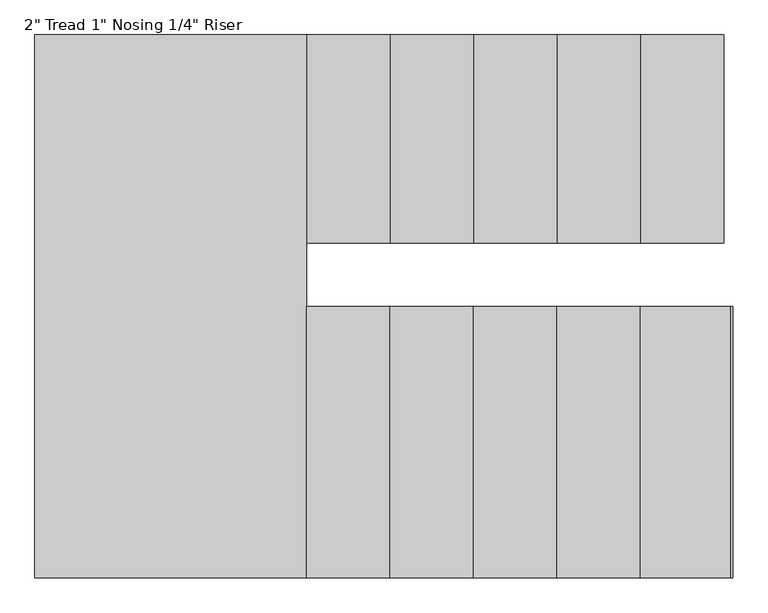
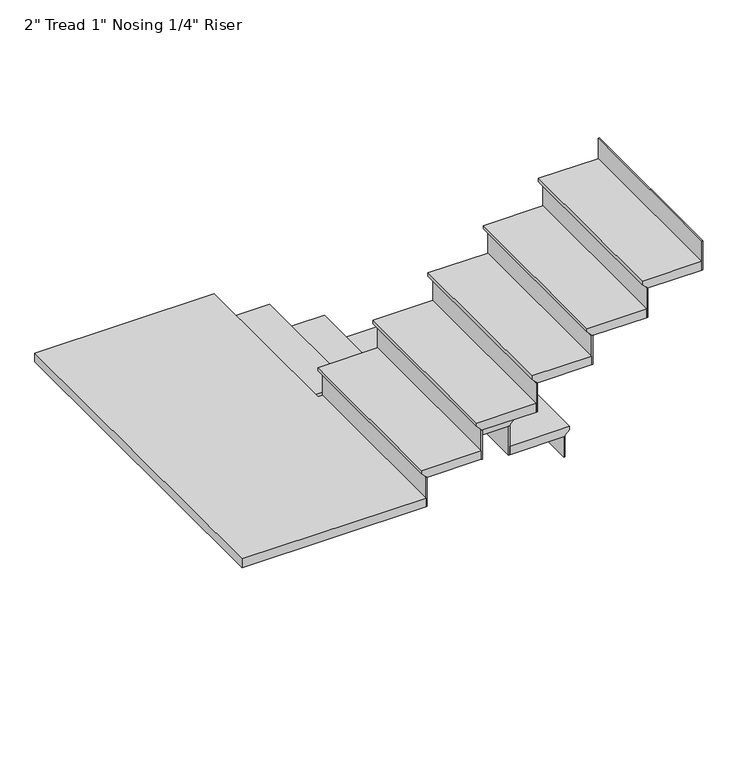
"""IFC4 building model written with IfcOpenShell, lengths in millimetres: stair flight geometry."""

from ifc_helpers import new_model, si_unit, origin, place, context, project, spatial, faceted_brep, source, transform, mapped, element, save


def stair_flight_99d63151(model_context):
    return source(origin(), model_context, "Body", "Brep", [
        faceted_brep([(-3084.0415084, -317.1427733, 9751.4833333), (-3084.0415084, -317.1427733, 9770.5333333), (-3084.0415084, -1076.6758739, 9770.5333333), (-3084.0415084, -1076.6758739, 9751.4833333), (-3109.4415084, -317.1427733, 9726.0833333), (-3109.4415084, -1076.6758739, 9726.0833333), (-3414.2415084, -317.1427733, 9770.5333333), (-3414.2415084, -1076.6758739, 9770.5333333), (-3109.4415084, -1076.6758739, 9719.7333333), (-3414.2415084, -1076.6758739, 9719.7333333), (-3414.2415084, -317.1427733, 9719.7333333), (-3109.4415084, -317.1427733, 9719.7333333)], [[[0, 1, 2, 3]], [[4, 0, 3, 5]], [[2, 1, 6, 7]], [[8, 9, 10, 11]], [[2, 7, 9, 8, 5, 3]], [[8, 11, 4, 5]], [[6, 1, 0, 4, 11, 10]], [[7, 6, 10, 9]]]),
        faceted_brep([(-3109.4415084, -317.1427733, 9719.7333333), (-3109.4415084, -317.1427733, 9601.2), (-3115.7915084, -317.1427733, 9601.2), (-3115.7915084, -317.1427733, 9719.7333333), (-3109.4415084, -1076.6758739, 9719.7333333), (-3115.7915084, -1076.6758739, 9719.7333333), (-3115.7915084, -1076.6758739, 9601.2), (-3109.4415084, -1076.6758739, 9601.2)], [[[0, 1, 2, 3]], [[4, 5, 6, 7]], [[1, 0, 4, 7]], [[2, 1, 7, 6]], [[3, 2, 6, 5]], [[0, 3, 5, 4]]]),
        faceted_brep([(-3414.2415084, -317.1427733, 9889.0666667), (-3414.2415084, -317.1427733, 9719.7333333), (-3420.5915084, -317.1427733, 9719.7333333), (-3420.5915084, -317.1427733, 9889.0666667), (-3414.2415084, -1076.6758739, 9889.0666667), (-3420.5915084, -1076.6758739, 9889.0666667), (-3420.5915084, -1076.6758739, 9719.7333333), (-3414.2415084, -1076.6758739, 9719.7333333)], [[[0, 1, 2, 3]], [[4, 5, 6, 7]], [[1, 0, 4, 7]], [[2, 1, 7, 6]], [[3, 2, 6, 5]], [[0, 3, 5, 4]]]),
        faceted_brep([(-3388.8415084, -1076.6758739, 9939.8666667), (-3388.8415084, -317.1427733, 9939.8666667), (-3719.0415084, -317.1427733, 9939.8666667), (-3719.0415084, -1076.6758739, 9939.8666667), (-3414.2415084, -1076.6758739, 9889.0666667), (-3719.0415084, -1076.6758739, 9889.0666667), (-3719.0415084, -317.1427733, 9889.0666667), (-3414.2415084, -317.1427733, 9889.0666667), (-3414.2415084, -1076.6758739, 9895.4166667), (-3388.8415084, -1076.6758739, 9920.8166667), (-3414.2415084, -317.1427733, 9895.4166667), (-3388.8415084, -317.1427733, 9920.8166667)], [[[0, 1, 2, 3]], [[4, 5, 6, 7]], [[0, 3, 5, 4, 8, 9]], [[4, 7, 10, 8]], [[2, 1, 11, 10, 7, 6]], [[3, 2, 6, 5]], [[11, 1, 0, 9]], [[10, 11, 9, 8]]]),
        faceted_brep([(-3719.0415084, -317.1427733, 10058.4), (-3719.0415084, -317.1427733, 9889.0666667), (-3725.3915084, -317.1427733, 9889.0666667), (-3725.3915084, -317.1427733, 10058.4), (-3719.0415084, -1076.6758739, 10058.4), (-3725.3915084, -1076.6758739, 10058.4), (-3725.3915084, -1076.6758739, 9889.0666667), (-3719.0415084, -1076.6758739, 9889.0666667)], [[[0, 1, 2, 3]], [[4, 5, 6, 7]], [[1, 0, 4, 7]], [[2, 1, 7, 6]], [[3, 2, 6, 5]], [[0, 3, 5, 4]]]),
        faceted_brep([(-3693.6415084, -1076.6758739, 10109.2), (-3693.6415084, -317.1427733, 10109.2), (-4023.8415084, -317.1427733, 10109.2), (-4023.8415084, -1076.6758739, 10109.2), (-3719.0415084, -1076.6758739, 10058.4), (-4023.8415084, -1076.6758739, 10058.4), (-4023.8415084, -317.1427733, 10058.4), (-3719.0415084, -317.1427733, 10058.4), (-3719.0415084, -1076.6758739, 10064.75), (-3693.6415084, -1076.6758739, 10090.15), (-3719.0415084, -317.1427733, 10064.75), (-3693.6415084, -317.1427733, 10090.15)], [[[0, 1, 2, 3]], [[4, 5, 6, 7]], [[0, 3, 5, 4, 8, 9]], [[4, 7, 10, 8]], [[2, 1, 11, 10, 7, 6]], [[3, 2, 6, 5]], [[11, 1, 0, 9]], [[10, 11, 9, 8]]]),
        faceted_brep([(-4023.8415084, -317.1427733, 10227.7333333), (-4023.8415084, -317.1427733, 10058.4), (-4030.1915084, -317.1427733, 10058.4), (-4030.1915084, -317.1427733, 10227.7333333), (-4023.8415084, -1076.6758739, 10227.7333333), (-4030.1915084, -1076.6758739, 10227.7333333), (-4030.1915084, -1076.6758739, 10058.4), (-4023.8415084, -1076.6758739, 10058.4)], [[[0, 1, 2, 3]], [[4, 5, 6, 7]], [[1, 0, 4, 7]], [[2, 1, 7, 6]], [[3, 2, 6, 5]], [[0, 3, 5, 4]]]),
        faceted_brep([(-3998.4415084, -1076.6758739, 10278.5333333), (-3998.4415084, -317.1427733, 10278.5333333), (-4328.6415084, -317.1427733, 10278.5333333), (-4328.6415084, -1076.6758739, 10278.5333333), (-4023.8415084, -1076.6758739, 10227.7333333), (-4328.6415084, -1076.6758739, 10227.7333333), (-4328.6415084, -317.1427733, 10227.7333333), (-4023.8415084, -317.1427733, 10227.7333333), (-4023.8415084, -1076.6758739, 10234.0833333), (-3998.4415084, -1076.6758739, 10259.4833333), (-4023.8415084, -317.1427733, 10234.0833333), (-3998.4415084, -317.1427733, 10259.4833333)], [[[0, 1, 2, 3]], [[4, 5, 6, 7]], [[0, 3, 5, 4, 8, 9]], [[4, 7, 10, 8]], [[2, 1, 11, 10, 7, 6]], [[3, 2, 6, 5]], [[11, 1, 0, 9]], [[10, 11, 9, 8]]]),
        faceted_brep([(-4328.6415084, -317.1427733, 10397.0666667), (-4328.6415084, -317.1427733, 10227.7333333), (-4334.9915084, -317.1427733, 10227.7333333), (-4334.9915084, -317.1427733, 10397.0666667), (-4328.6415084, -1076.6758739, 10397.0666667), (-4334.9915084, -1076.6758739, 10397.0666667), (-4334.9915084, -1076.6758739, 10227.7333333), (-4328.6415084, -1076.6758739, 10227.7333333)], [[[0, 1, 2, 3]], [[4, 5, 6, 7]], [[1, 0, 4, 7]], [[2, 1, 7, 6]], [[3, 2, 6, 5]], [[0, 3, 5, 4]]]),
        faceted_brep([(-4303.2415084, -1076.6758739, 10447.8666667), (-4303.2415084, -317.1427733, 10447.8666667), (-4633.4415084, -317.1427733, 10447.8666667), (-4633.4415084, -1076.6758739, 10447.8666667), (-4328.6415084, -1076.6758739, 10397.0666667), (-4633.4415084, -1076.6758739, 10397.0666667), (-4633.4415084, -317.1427733, 10397.0666667), (-4328.6415084, -317.1427733, 10397.0666667), (-4328.6415084, -1076.6758739, 10403.4166667), (-4303.2415084, -1076.6758739, 10428.8166667), (-4328.6415084, -317.1427733, 10403.4166667), (-4303.2415084, -317.1427733, 10428.8166667)], [[[0, 1, 2, 3]], [[4, 5, 6, 7]], [[0, 3, 5, 4, 8, 9]], [[4, 7, 10, 8]], [[2, 1, 11, 10, 7, 6]], [[3, 2, 6, 5]], [[11, 1, 0, 9]], [[10, 11, 9, 8]]]),
        faceted_brep([(-4633.4415084, -317.1427733, 10566.4), (-4633.4415084, -317.1427733, 10397.0666667), (-4639.7915084, -317.1427733, 10397.0666667), (-4639.7915084, -317.1427733, 10566.4), (-4633.4415084, -1076.6758739, 10566.4), (-4639.7915084, -1076.6758739, 10566.4), (-4639.7915084, -1076.6758739, 10397.0666667), (-4633.4415084, -1076.6758739, 10397.0666667)], [[[0, 1, 2, 3]], [[4, 5, 6, 7]], [[1, 0, 4, 7]], [[2, 1, 7, 6]], [[3, 2, 6, 5]], [[0, 3, 5, 4]]]),
        faceted_brep([(-4582.6415084, -1307.7427733, 10617.2), (-4608.0415084, -1307.7427733, 10617.2), (-4608.0415084, -317.1427733, 10617.2), (-5598.6415084, -317.1427733, 10617.2), (-5598.6415084, -2298.3427733, 10617.2), (-4582.6415084, -2298.3427733, 10617.2), (-4608.0415084, -1307.7427733, 10566.4), (-4582.6415084, -1307.7427733, 10566.4), (-4582.6415084, -2298.3427733, 10566.4), (-5598.6415084, -2298.3427733, 10566.4), (-5598.6415084, -317.1427733, 10566.4), (-4633.4415084, -317.1427733, 10566.4), (-4633.4415084, -1076.6758739, 10566.4), (-4608.0415084, -1076.6758739, 10566.4), (-4608.0415084, -1076.6758739, 10598.15), (-4608.0415084, -317.1427733, 10598.15), (-4633.4415084, -1076.6758739, 10572.75), (-4633.4415084, -317.1427733, 10572.75)], [[[0, 1, 2, 3, 4, 5]], [[6, 7, 8, 9, 10, 11, 12, 13]], [[1, 0, 7, 6]], [[2, 1, 6, 13, 14, 15]], [[13, 12, 16, 14]], [[12, 11, 17, 16]], [[3, 2, 15, 17, 11, 10]], [[4, 3, 10, 9]], [[5, 4, 9, 8]], [[0, 5, 8, 7]], [[17, 15, 14, 16]]]),
        faceted_brep([(-4582.6415084, -2298.3427733, 10735.7333333), (-4582.6415084, -2298.3427733, 10566.4), (-4576.2915084, -2298.3427733, 10566.4), (-4576.2915084, -2298.3427733, 10735.7333333), (-4582.6415084, -1307.7427733, 10735.7333333), (-4576.2915084, -1307.7427733, 10735.7333333), (-4576.2915084, -1307.7427733, 10566.4), (-4582.6415084, -1307.7427733, 10566.4)], [[[0, 1, 2, 3]], [[4, 5, 6, 7]], [[1, 0, 4, 7]], [[2, 1, 7, 6]], [[3, 2, 6, 5]], [[0, 3, 5, 4]]]),
        faceted_brep([(-4608.0415084, -1307.7427733, 10786.5333333), (-4608.0415084, -2298.3427733, 10786.5333333), (-4277.8415084, -2298.3427733, 10786.5333333), (-4277.8415084, -1307.7427733, 10786.5333333), (-4582.6415084, -1307.7427733, 10735.7333333), (-4277.8415084, -1307.7427733, 10735.7333333), (-4277.8415084, -2298.3427733, 10735.7333333), (-4582.6415084, -2298.3427733, 10735.7333333), (-4582.6415084, -1307.7427733, 10742.0833333), (-4608.0415084, -1307.7427733, 10767.4833333), (-4582.6415084, -2298.3427733, 10742.0833333), (-4608.0415084, -2298.3427733, 10767.4833333)], [[[0, 1, 2, 3]], [[4, 5, 6, 7]], [[0, 3, 5, 4, 8, 9]], [[4, 7, 10, 8]], [[2, 1, 11, 10, 7, 6]], [[3, 2, 6, 5]], [[11, 1, 0, 9]], [[10, 11, 9, 8]]]),
        faceted_brep([(-4277.8415084, -2298.3427733, 10905.0666667), (-4277.8415084, -2298.3427733, 10735.7333333), (-4271.4915084, -2298.3427733, 10735.7333333), (-4271.4915084, -2298.3427733, 10905.0666667), (-4277.8415084, -1307.7427733, 10905.0666667), (-4271.4915084, -1307.7427733, 10905.0666667), (-4271.4915084, -1307.7427733, 10735.7333333), (-4277.8415084, -1307.7427733, 10735.7333333)], [[[0, 1, 2, 3]], [[4, 5, 6, 7]], [[1, 0, 4, 7]], [[2, 1, 7, 6]], [[3, 2, 6, 5]], [[0, 3, 5, 4]]]),
        faceted_brep([(-4303.2415084, -1307.7427733, 10955.8666667), (-4303.2415084, -2298.3427733, 10955.8666667), (-3973.0415084, -2298.3427733, 10955.8666667), (-3973.0415084, -1307.7427733, 10955.8666667), (-4277.8415084, -1307.7427733, 10905.0666667), (-3973.0415084, -1307.7427733, 10905.0666667), (-3973.0415084, -2298.3427733, 10905.0666667), (-4277.8415084, -2298.3427733, 10905.0666667), (-4277.8415084, -1307.7427733, 10911.4166667), (-4303.2415084, -1307.7427733, 10936.8166667), (-4277.8415084, -2298.3427733, 10911.4166667), (-4303.2415084, -2298.3427733, 10936.8166667)], [[[0, 1, 2, 3]], [[4, 5, 6, 7]], [[0, 3, 5, 4, 8, 9]], [[4, 7, 10, 8]], [[2, 1, 11, 10, 7, 6]], [[3, 2, 6, 5]], [[11, 1, 0, 9]], [[10, 11, 9, 8]]]),
        faceted_brep([(-3973.0415084, -2298.3427733, 11074.4), (-3973.0415084, -2298.3427733, 10905.0666667), (-3966.6915084, -2298.3427733, 10905.0666667), (-3966.6915084, -2298.3427733, 11074.4), (-3973.0415084, -1307.7427733, 11074.4), (-3966.6915084, -1307.7427733, 11074.4), (-3966.6915084, -1307.7427733, 10905.0666667), (-3973.0415084, -1307.7427733, 10905.0666667)], [[[0, 1, 2, 3]], [[4, 5, 6, 7]], [[1, 0, 4, 7]], [[2, 1, 7, 6]], [[3, 2, 6, 5]], [[0, 3, 5, 4]]]),
        faceted_brep([(-3998.4415084, -1307.7427733, 11125.2), (-3998.4415084, -2298.3427733, 11125.2), (-3668.2415084, -2298.3427733, 11125.2), (-3668.2415084, -1307.7427733, 11125.2), (-3973.0415084, -1307.7427733, 11074.4), (-3668.2415084, -1307.7427733, 11074.4), (-3668.2415084, -2298.3427733, 11074.4), (-3973.0415084, -2298.3427733, 11074.4), (-3973.0415084, -1307.7427733, 11080.75), (-3998.4415084, -1307.7427733, 11106.15), (-3973.0415084, -2298.3427733, 11080.75), (-3998.4415084, -2298.3427733, 11106.15)], [[[0, 1, 2, 3]], [[4, 5, 6, 7]], [[0, 3, 5, 4, 8, 9]], [[4, 7, 10, 8]], [[2, 1, 11, 10, 7, 6]], [[3, 2, 6, 5]], [[11, 1, 0, 9]], [[10, 11, 9, 8]]]),
        faceted_brep([(-3668.2415084, -2298.3427733, 11243.7333333), (-3668.2415084, -2298.3427733, 11074.4), (-3661.8915084, -2298.3427733, 11074.4), (-3661.8915084, -2298.3427733, 11243.7333333), (-3668.2415084, -1307.7427733, 11243.7333333), (-3661.8915084, -1307.7427733, 11243.7333333), (-3661.8915084, -1307.7427733, 11074.4), (-3668.2415084, -1307.7427733, 11074.4)], [[[0, 1, 2, 3]], [[4, 5, 6, 7]], [[1, 0, 4, 7]], [[2, 1, 7, 6]], [[3, 2, 6, 5]], [[0, 3, 5, 4]]]),
        faceted_brep([(-3693.6415084, -1307.7427733, 11294.5333333), (-3693.6415084, -2298.3427733, 11294.5333333), (-3363.4415084, -2298.3427733, 11294.5333333), (-3363.4415084, -1307.7427733, 11294.5333333), (-3668.2415084, -1307.7427733, 11243.7333333), (-3363.4415084, -1307.7427733, 11243.7333333), (-3363.4415084, -2298.3427733, 11243.7333333), (-3668.2415084, -2298.3427733, 11243.7333333), (-3668.2415084, -1307.7427733, 11250.0833333), (-3693.6415084, -1307.7427733, 11275.4833333), (-3668.2415084, -2298.3427733, 11250.0833333), (-3693.6415084, -2298.3427733, 11275.4833333)], [[[0, 1, 2, 3]], [[4, 5, 6, 7]], [[0, 3, 5, 4, 8, 9]], [[4, 7, 10, 8]], [[2, 1, 11, 10, 7, 6]], [[3, 2, 6, 5]], [[11, 1, 0, 9]], [[10, 11, 9, 8]]]),
        faceted_brep([(-3363.4415084, -2298.3427733, 11413.0666667), (-3363.4415084, -2298.3427733, 11243.7333333), (-3357.0915084, -2298.3427733, 11243.7333333), (-3357.0915084, -2298.3427733, 11413.0666667), (-3363.4415084, -1307.7427733, 11413.0666667), (-3357.0915084, -1307.7427733, 11413.0666667), (-3357.0915084, -1307.7427733, 11243.7333333), (-3363.4415084, -1307.7427733, 11243.7333333)], [[[0, 1, 2, 3]], [[4, 5, 6, 7]], [[1, 0, 4, 7]], [[2, 1, 7, 6]], [[3, 2, 6, 5]], [[0, 3, 5, 4]]]),
        faceted_brep([(-3058.6415084, -2298.3427733, 11582.4), (-3058.6415084, -2298.3427733, 11413.0666667), (-3052.2915084, -2298.3427733, 11413.0666667), (-3052.2915084, -2298.3427733, 11582.4), (-3058.6415084, -1307.7427733, 11582.4), (-3052.2915084, -1307.7427733, 11582.4), (-3052.2915084, -1307.7427733, 11413.0666667), (-3058.6415084, -1307.7427733, 11413.0666667)], [[[0, 1, 2, 3]], [[4, 5, 6, 7]], [[1, 0, 4, 7]], [[2, 1, 7, 6]], [[3, 2, 6, 5]], [[0, 3, 5, 4]]]),
        faceted_brep([(-3388.8415084, -1307.7427733, 11463.8666667), (-3388.8415084, -2298.3427733, 11463.8666667), (-3058.6415084, -2298.3427733, 11463.8666667), (-3058.6415084, -1307.7427733, 11463.8666667), (-3363.4415084, -1307.7427733, 11413.0666667), (-3058.6415084, -1307.7427733, 11413.0666667), (-3058.6415084, -2298.3427733, 11413.0666667), (-3363.4415084, -2298.3427733, 11413.0666667), (-3363.4415084, -1307.7427733, 11419.4166667), (-3388.8415084, -1307.7427733, 11444.8166667), (-3363.4415084, -2298.3427733, 11419.4166667), (-3388.8415084, -2298.3427733, 11444.8166667)], [[[0, 1, 2, 3]], [[4, 5, 6, 7]], [[0, 3, 5, 4, 8, 9]], [[4, 7, 10, 8]], [[2, 1, 11, 10, 7, 6]], [[3, 2, 6, 5]], [[11, 1, 0, 9]], [[10, 11, 9, 8]]]),
    ])


if __name__ == "__main__":
    model = new_model("IFC4")
    model_context = context("Model", 3, world=origin())
    ifc_project = project(units=[si_unit("LENGTHUNIT", "METRE", prefix="MILLI")], contexts=[model_context])
    site = spatial("IfcSite", under=ifc_project)
    building = spatial("IfcBuilding", under=site)
    placement = place(None, origin())
    stair_flight_shape = stair_flight_99d63151(model_context)
    element("IfcStairFlight", 1, ObjectType="2\" Tread 1\" Nosing 1/4\" Riser", at=placement, inside=building, context=model_context, shape_type="MappedRepresentation", body=[
        mapped(stair_flight_shape, transform((0.0, 0.0, 0.0), x_axis=(1.0, 0.0, 0.0), y_axis=(0.0, 1.0, 0.0), z_axis=(0.0, 0.0, 1.0))),
    ])
    save(model, "model.ifc")
